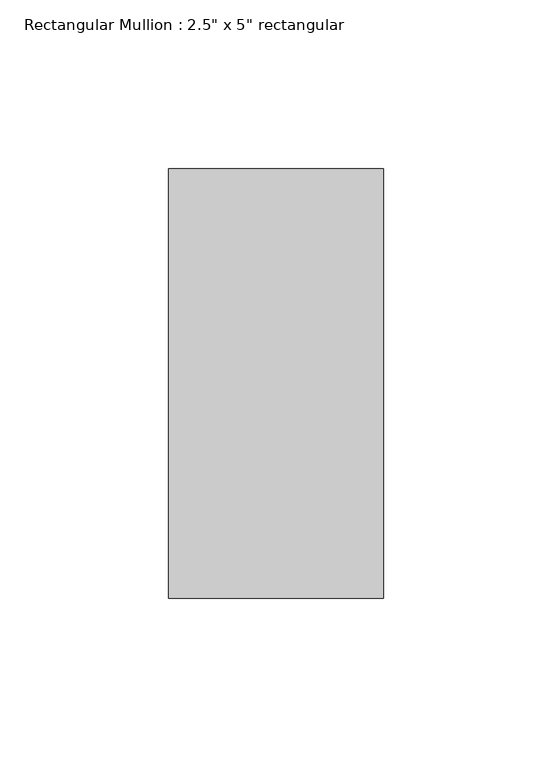
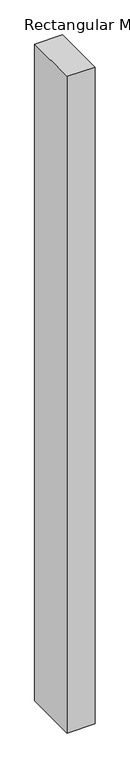
"""IFC4 building model written with IfcOpenShell, lengths in millimetres: member geometry."""

from ifc_helpers import new_model, si_unit, frame, origin, place, context, project, spatial, polyline, outline, extrude, source, transform, mapped, element, save


def member_6ce1ec76(model_context):
    return source(origin(), model_context, "Body", "SweptSolid", [
        extrude(outline(polyline([(0.0, 63.5), (0.0, -63.5), (-63.5, -63.5), (-63.5, 63.5), (0.0, 63.5)])), frame((0.0, 0.0, -1574.8), z_axis=(0.0, 0.0, 1.0), x_axis=(1.0, 0.0, 0.0)), (0.0, 0.0, 1.0), 1574.8),
    ])


if __name__ == "__main__":
    model = new_model("IFC4")
    model_context = context("Model", 3, world=origin())
    ifc_project = project(units=[si_unit("LENGTHUNIT", "METRE", prefix="MILLI")], contexts=[model_context])
    site = spatial("IfcSite", under=ifc_project)
    building = spatial("IfcBuilding", under=site)
    placement = place(None, origin())
    member_shape = member_6ce1ec76(model_context)
    element("IfcMember", 1, ObjectType="Rectangular Mullion : 2.5\" x 5\" rectangular", at=placement, inside=building, context=model_context, shape_type="MappedRepresentation", body=[
        mapped(member_shape, transform((0.0, 0.0, 0.0), x_axis=(1.0, 0.0, 0.0), y_axis=(0.0, 1.0, 0.0), z_axis=(0.0, 0.0, 1.0))),
    ])
    save(model, "model.ifc")

# Revit data of these elements
# Type "Rectangular Mullion : 2.5\" x 5\" rectangular"
#   built-in parameter 1007304 = 0.416667 (stored number, unit not read)
#   built-in parameter 1007301 = 0.104167 (stored number, unit not read)
#   built-in parameter 1007300 = 0.104167 (stored number, unit not read)
# Element 1 (IfcMember, "Rectangular Mullion : 2.5\" x 5\" rectangular")
#   Materials on its faces: "Aluminum"
# Materials
#   "Aluminum": class "Metal", colour RGB 247 247 247, transparency 0, Description = "Aluminum 6061", Cost = 0
